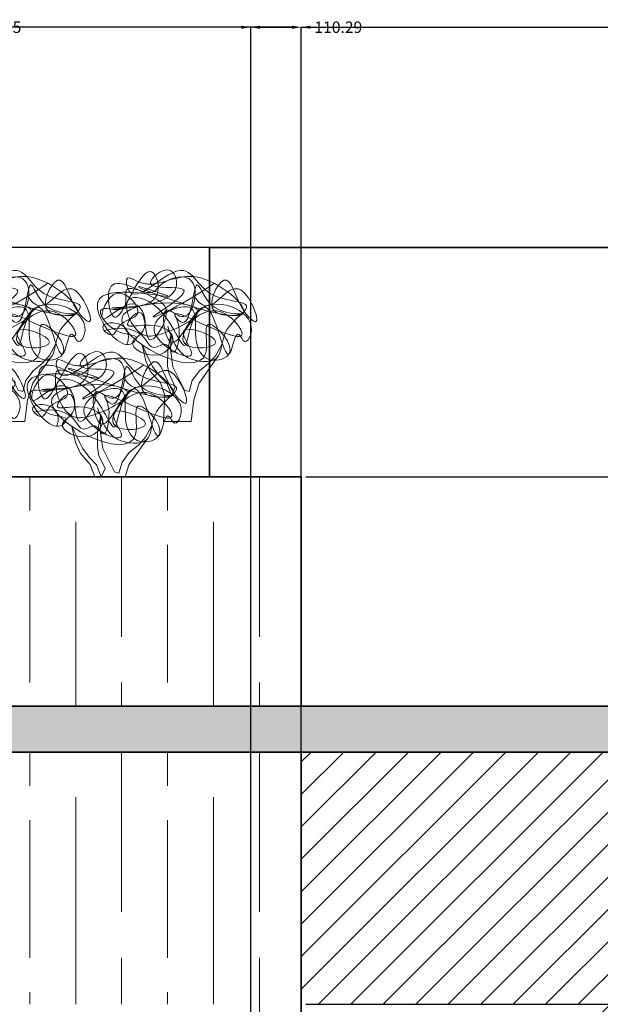
# Model space of a CAD drawing. Units: millimetres. Extents: x -692 to 9639, y -141 to 10345.
# Tile 17 of 19: x 4578 to 5843, y 8199 to 10345. Entities that reach past the tile are written whole.
import ezdxf

# ---------------------------------------------------------------- set-up
doc = ezdxf.new("R2010")
doc.units = ezdxf.units.MM
doc.header["$MEASUREMENT"] = 0
for name, color, linetype, lineweight in [('A-ANNO-DIMS', 2, 'Continuous', 18), ('A-ELEV', 7, 'Continuous', 35), ('A-ELEV-PATT', 8, 'Continuous', 13), ('L-PLNT', 3, 'Continuous', 18)]:
    doc.layers.add(name, color=color, linetype=linetype, lineweight=lineweight)
doc.styles.get("Standard").update_dxf_attribs({"font": 'arial.ttf'})
doc.dimstyles.get("Standard").update_dxf_attribs({"dimtxt": 25, "dimasz": 20, "dimexe": 0.18, "dimexo": 10, "dimgap": 10, "dimtad": 0, "dimtih": 1, "dimtoh": 1, "dimdec": 0, "dimzin": 0, "dimdsep": 46, "dimtxsty": 'Standard', "dimcen": 10, "dimadec": 0, "dimazin": 0, "dimtfac": 1, "dimtdec": 0, "dimtofl": 0, "dimtmove": 0, "dimatfit": 3, "dimfxl": 1, "dimtolj": 1, "dimtzin": 0, "dimarcsym": 0})

# ---------------------------------------------------------------- blocks, each defined once
blk = doc.blocks.new('SHRUB-A')
for p, q in [((56.2, 156.7), (63.1, 192.4)), ((63.1, 192.4), (61.6, 157.6)), ((4.3, 148.6), (0, 167.6)), ((0, 167.6), (10, 146.8)), ((55.6, 120.9), (56.2, 156.7)), ((61.6, 157.6), (67.3, 119.6)), ((160.6, 144.2), (174.3, 169.5)), ((7.9, 132.5), (4.3, 148.6)), ((17.8, 109.9), (7.9, 132.5)), ((10, 146.8), (18, 130.3)), ((18, 130.3), (22.9, 120.3)), ((162.4, 138.4), (124.4, 83.7)), ((145.1, 126.5), (160.6, 144.2)), ((40.2, 84.8), (17.8, 109.9)), ((22.9, 120.3), (37.4, 100.1)), ((59.1, 104.1), (55.6, 120.9)), ((67.3, 119.6), (83.9, 86)), ((109.4, 89.7), (124.8, 110.5)), ((124.8, 110.5), (145.1, 126.5)), ((37.4, 100.1), (54, 83.6)), ((72.4, 75.8), (59.1, 104.1)), ((83.9, 86), (92.7, 68.2)), ((102.6, 65.4), (109.4, 89.7)), ((49.7, 57.7), (40.2, 84.8)), ((54, 83.6), (64.1, 57.4)), ((64.1, 57.4), (72.4, 75.8)), ((92.7, 68.2), (102.6, 65.4)), ((124.4, 83.7), (113, 47.4)), ((47, 0.4), (49.7, 57.7)), ((113, 47.4), (106.7, 0)), ((106.7, 0), (47, 0.4))]:
    blk.add_line(p, q)
blk = doc.blocks.new('SHRUB-B')
for p, q in [((56.2, 99.2), (63.1, 135)), ((63.1, 135), (61.6, 100.2)), ((4.3, 91.2), (0, 110.2)), ((0, 110.2), (10, 89.4)), ((160.6, 86.8), (174.3, 112.1)), ((7.9, 75.1), (4.3, 91.2)), ((10, 89.4), (18, 72.9)), ((55.6, 63.5), (56.2, 99.2)), ((61.6, 100.2), (67.3, 62.2)), ((145.1, 69.1), (160.6, 86.8)), ((17.8, 52.5), (7.9, 75.1)), ((18, 72.9), (22.9, 62.9)), ((124.8, 53.1), (145.1, 69.1)), ((40.2, 27.4), (17.8, 52.5)), ((22.9, 62.9), (37.4, 42.7)), ((59.1, 46.7), (55.6, 63.5)), ((72.4, 18.4), (59.1, 46.7)), ((67.3, 62.2), (83.9, 28.6)), ((109.4, 32.3), (124.8, 53.1)), ((37.4, 42.7), (54, 26.2)), ((49.7, 0.3), (40.2, 27.4)), ((54, 26.2), (64.1, 0)), ((83.9, 28.6), (92.7, 10.8)), ((102.6, 8), (109.4, 32.3)), ((64.1, 0), (72.4, 18.4)), ((92.7, 10.8), (102.6, 8))]:
    blk.add_line(p, q)
blk = doc.blocks.new('*D7')
at = {"layer": 'A-ANNO-DIMS', "color": 0, "lineweight": -2, "transparency": 16777216}
for p, q in [((8481.5, 9848.8), (-649.1, 9848.8)), ((-648.9, 9828.8), (-648.9, 5124.9)), ((-648.9, 375.6), (-648.9, 5079.4)), ((2463.7, 355.6), (-649.1, 355.6))]:
    blk.add_line(p, q, dxfattribs=at)
at = {"layer": 'A-ANNO-DIMS', "color": 0, "lineweight": -3, "transparency": 16777216}
for points in [[(-652.2, 9828.8), (-645.6, 9828.8), (-648.9, 9848.8)], [(-652.2, 375.6), (-645.6, 375.6), (-648.9, 355.6)]]:
    blk.add_solid(points, dxfattribs=at)
at = {"layer": 'Defpoints', "color": 0, "lineweight": -3, "transparency": 16777216}
for p in [(-648.9, 9848.8), (8491.5, 9848.8), (2473.7, 355.6)]:
    blk.add_point(p, dxfattribs=at)
at = {"layer": 'A-ANNO-DIMS', "color": 0, "transparency": 16777216, "insert": (-648.9, 5102.2), "char_height": 25, "attachment_point": 5}
blk.add_mtext('\\A1;9493', dxfattribs=at)
blk = doc.blocks.new('*D11')
at = {"layer": 'A-ANNO-DIMS', "color": 0, "lineweight": -2, "transparency": 16777216}
for p, q in [((9553.7, 9348.8), (9553.7, 9368.8)), ((9553.7, 9368.8), (9573.7, 9368.8)), ((5201.5, 9348.8), (9553.9, 9348.8)), ((9553.7, 9268.8), (9553.7, 9328.8)), ((8251.5, 9248.8), (9553.9, 9248.8))]:
    blk.add_line(p, q, dxfattribs=at)
at = {"layer": 'A-ANNO-DIMS', "color": 0, "lineweight": -3, "transparency": 16777216}
for points in [[(9550.4, 9328.8), (9557.1, 9328.8), (9553.7, 9348.8)], [(9550.4, 9268.8), (9557.1, 9268.8), (9553.7, 9248.8)]]:
    blk.add_solid(points, dxfattribs=at)
at = {"layer": 'Defpoints', "color": 0, "lineweight": -3, "transparency": 16777216}
for p in [(5191.5, 9348.8), (9553.7, 9348.8), (8241.5, 9248.8)]:
    blk.add_point(p, dxfattribs=at)
at = {"layer": 'A-ANNO-DIMS', "color": 0, "transparency": 16777216, "insert": (9610.1, 9368.8), "char_height": 25, "attachment_point": 5}
blk.add_mtext('\\A1;100', dxfattribs=at)
blk = doc.blocks.new('*D12')
at = {"layer": 'A-ANNO-DIMS', "color": 0, "lineweight": -2, "transparency": 16777216}
for p, q in [((8251.5, 9598.8), (9553.9, 9598.8)), ((9553.7, 9578.8), (9553.7, 9496.5)), ((9553.7, 9368.8), (9553.7, 9451)), ((5201.5, 9348.8), (9553.9, 9348.8))]:
    blk.add_line(p, q, dxfattribs=at)
at = {"layer": 'A-ANNO-DIMS', "color": 0, "lineweight": -3, "transparency": 16777216}
for points in [[(9550.4, 9578.8), (9557.1, 9578.8), (9553.7, 9598.8)], [(9550.4, 9368.8), (9557.1, 9368.8), (9553.7, 9348.8)]]:
    blk.add_solid(points, dxfattribs=at)
at = {"layer": 'Defpoints', "color": 0, "lineweight": -3, "transparency": 16777216}
for p in [(8241.5, 9598.8), (9553.7, 9598.8), (5191.5, 9348.8)]:
    blk.add_point(p, dxfattribs=at)
at = {"layer": 'A-ANNO-DIMS', "color": 0, "transparency": 16777216, "insert": (9553.7, 9473.8), "char_height": 25, "attachment_point": 5}
blk.add_mtext('\\A1;250', dxfattribs=at)
blk = doc.blocks.new('*D14')
at = {"layer": 'A-ANNO-DIMS', "color": 0, "lineweight": -2, "transparency": 16777216}
for p, q in [((3191.5, 9358.8), (3191.5, 10329)), ((3211.5, 10328.8), (4144, 10328.8)), ((5171.5, 10328.8), (4239, 10328.8)), ((5191.5, 9358.8), (5191.5, 10329))]:
    blk.add_line(p, q, dxfattribs=at)
at = {"layer": 'A-ANNO-DIMS', "color": 0, "lineweight": -3, "transparency": 16777216}
for points in [[(3211.5, 10332.1), (3211.5, 10325.4), (3191.5, 10328.8)], [(5171.5, 10332.1), (5171.5, 10325.4), (5191.5, 10328.8)]]:
    blk.add_solid(points, dxfattribs=at)
at = {"layer": 'Defpoints', "color": 0, "lineweight": -3, "transparency": 16777216}
for p in [(5191.5, 10328.8), (3191.5, 9348.8), (5191.5, 9348.8)]:
    blk.add_point(p, dxfattribs=at)
at = {"layer": 'A-ANNO-DIMS', "color": 0, "transparency": 16777216, "insert": (4191.5, 10328.8), "char_height": 25, "attachment_point": 5}
blk.add_mtext('\\A1;2000', dxfattribs=at)
blk = doc.blocks.new('*D15')
at = {"layer": 'A-ANNO-DIMS', "color": 0, "lineweight": -2, "transparency": 16777216}
for p, q in [((5191.5, 9358.8), (5191.5, 10329)), ((5211.5, 10328.8), (5920.4, 10328.8)), ((6721.5, 10328.8), (6012.7, 10328.8)), ((6741.5, 9258.8), (6741.5, 10329))]:
    blk.add_line(p, q, dxfattribs=at)
at = {"layer": 'A-ANNO-DIMS', "color": 0, "lineweight": -3, "transparency": 16777216}
for points in [[(5211.5, 10332.1), (5211.5, 10325.4), (5191.5, 10328.8)], [(6721.5, 10332.1), (6721.5, 10325.4), (6741.5, 10328.8)]]:
    blk.add_solid(points, dxfattribs=at)
at = {"layer": 'Defpoints', "color": 0, "lineweight": -3, "transparency": 16777216}
for p in [(6741.5, 10328.8), (5191.5, 9348.8), (6741.5, 9248.8)]:
    blk.add_point(p, dxfattribs=at)
at = {"layer": 'A-ANNO-DIMS', "color": 0, "transparency": 16777216, "insert": (5966.5, 10328.8), "char_height": 25, "attachment_point": 5}
blk.add_mtext('\\A1;1550', dxfattribs=at)
blk = doc.blocks.new('*D54')
at = {"layer": 'A-ANNO-DIMS', "color": 0, "lineweight": -2, "transparency": 16777216}
for p, q in [((4006.3, 6433.8), (4006.3, 10329)), ((4026.3, 10328.8), (4497.5, 10328.8)), ((5061.3, 10328.8), (4590, 10328.8)), ((5081.3, 6433.8), (5081.3, 10329))]:
    blk.add_line(p, q, dxfattribs=at)
at = {"layer": 'A-ANNO-DIMS', "color": 0, "lineweight": -3, "transparency": 16777216}
for points in [[(4026.3, 10332.1), (4026.3, 10325.4), (4006.3, 10328.8)], [(5061.3, 10332.1), (5061.3, 10325.4), (5081.3, 10328.8)]]:
    blk.add_solid(points, dxfattribs=at)
at = {"layer": 'Defpoints', "color": 0, "lineweight": -3, "transparency": 16777216}
for p in [(5081.3, 10328.8), (4006.3, 6423.8), (5081.3, 6423.8)]:
    blk.add_point(p, dxfattribs=at)
at = {"layer": 'A-ANNO-DIMS', "color": 0, "transparency": 16777216, "insert": (4543.8, 10328.8), "char_height": 25, "attachment_point": 5}
blk.add_mtext('\\A1;1075', dxfattribs=at)
blk = doc.blocks.new('*D55')
at = {"layer": 'A-ANNO-DIMS', "color": 0, "lineweight": -2, "transparency": 16777216}
for p, q in [((5081.3, 6433.8), (5081.3, 10329)), ((5101.3, 10328.8), (5171.5, 10328.8)), ((5191.5, 6358.8), (5191.5, 10329)), ((5191.5, 10328.8), (5211.5, 10328.8))]:
    blk.add_line(p, q, dxfattribs=at)
at = {"layer": 'A-ANNO-DIMS', "color": 0, "lineweight": -3, "transparency": 16777216}
for points in [[(5101.3, 10332.1), (5101.3, 10325.4), (5081.3, 10328.8)], [(5171.5, 10332.1), (5171.5, 10325.4), (5191.5, 10328.8)]]:
    blk.add_solid(points, dxfattribs=at)
at = {"layer": 'Defpoints', "color": 0, "lineweight": -3, "transparency": 16777216}
for p in [(5191.5, 10328.8), (5081.3, 6423.8), (5191.5, 6348.8)]:
    blk.add_point(p, dxfattribs=at)
at = {"layer": 'A-ANNO-DIMS', "color": 0, "transparency": 16777216, "insert": (5272.3, 10328.8), "char_height": 25, "attachment_point": 5}
blk.add_mtext('\\A1;110.29', dxfattribs=at)
blk = doc.blocks.new('*D56')
at = {"layer": 'A-ANNO-DIMS', "color": 0, "lineweight": -2, "transparency": 16777216}
for p, q in [((5191.5, 6358.8), (5191.5, 10329)), ((5211.5, 10328.8), (5981.1, 10328.8)), ((6871.7, 10328.8), (6102.2, 10328.8)), ((6891.7, 6708.8), (6891.7, 10329))]:
    blk.add_line(p, q, dxfattribs=at)
at = {"layer": 'A-ANNO-DIMS', "color": 0, "lineweight": -3, "transparency": 16777216}
for points in [[(5211.5, 10332.1), (5211.5, 10325.4), (5191.5, 10328.8)], [(6871.7, 10332.1), (6871.7, 10325.4), (6891.7, 10328.8)]]:
    blk.add_solid(points, dxfattribs=at)
at = {"layer": 'Defpoints', "color": 0, "lineweight": -3, "transparency": 16777216}
for p in [(6891.7, 10328.8), (6891.7, 6698.8), (5191.5, 6348.8)]:
    blk.add_point(p, dxfattribs=at)
at = {"layer": 'A-ANNO-DIMS', "color": 0, "transparency": 16777216, "insert": (6041.6, 10328.8), "char_height": 25, "attachment_point": 5}
blk.add_mtext('\\A1;1700.2', dxfattribs=at)
blk = doc.blocks.new('*D77')
at = {"layer": 'A-ANNO-DIMS', "color": 0, "lineweight": -2, "transparency": 16777216}
for p, q in [((5201.5, 8198.8), (9553.9, 8198.8)), ((9553.7, 8178.8), (9553.7, 7771.8)), ((9553.7, 7319.3), (9553.7, 7726.3)), ((5201.5, 7299.3), (9553.9, 7299.3))]:
    blk.add_line(p, q, dxfattribs=at)
at = {"layer": 'A-ANNO-DIMS', "color": 0, "lineweight": -3, "transparency": 16777216}
for points in [[(9550.4, 8178.8), (9557.1, 8178.8), (9553.7, 8198.8)], [(9550.4, 7319.3), (9557.1, 7319.3), (9553.7, 7299.3)]]:
    blk.add_solid(points, dxfattribs=at)
at = {"layer": 'Defpoints', "color": 0, "lineweight": -3, "transparency": 16777216}
for p in [(5191.5, 8198.8), (9553.7, 8198.8), (5191.5, 7299.3)]:
    blk.add_point(p, dxfattribs=at)
at = {"layer": 'A-ANNO-DIMS', "color": 0, "transparency": 16777216, "insert": (9553.7, 7749), "char_height": 25, "attachment_point": 5}
blk.add_mtext('\\A1;899.5', dxfattribs=at)
blk = doc.blocks.new('*D78')
at = {"layer": 'A-ANNO-DIMS', "color": 0, "lineweight": -2, "transparency": 16777216}
for p, q in [((8401.5, 8748.8), (9553.9, 8748.8)), ((9553.7, 8728.8), (9553.7, 8496.5)), ((9553.7, 8218.8), (9553.7, 8451)), ((5201.5, 8198.8), (9553.9, 8198.8))]:
    blk.add_line(p, q, dxfattribs=at)
at = {"layer": 'A-ANNO-DIMS', "color": 0, "lineweight": -3, "transparency": 16777216}
for points in [[(9550.4, 8728.8), (9557.1, 8728.8), (9553.7, 8748.8)], [(9550.4, 8218.8), (9557.1, 8218.8), (9553.7, 8198.8)]]:
    blk.add_solid(points, dxfattribs=at)
at = {"layer": 'Defpoints', "color": 0, "lineweight": -3, "transparency": 16777216}
for p in [(8391.5, 8748.8), (9553.7, 8748.8), (5191.5, 8198.8)]:
    blk.add_point(p, dxfattribs=at)
at = {"layer": 'A-ANNO-DIMS', "color": 0, "transparency": 16777216, "insert": (9553.7, 8473.8), "char_height": 25, "attachment_point": 5}
blk.add_mtext('\\A1;550', dxfattribs=at)

msp = doc.modelspace()

# ---------------------------------------------------------------- hatches: boundary and pattern name
at = {"layer": 'A-ELEV-PATT'}
h = msp.add_hatch(dxfattribs=at)
h.set_pattern_fill('GOST_WOOD', color=256, scale=50)
h.set_pattern_definition([(90, (0, 0), (300, -2e-14), [500, -100]), (90, (100, -100), (300, -2e-14), [300, -75, 150, -75]), (90, (200, -250), (300, -2e-14), [500, -100])])
edge = h.paths.add_edge_path()
edge.add_line((5191.547, 8748.772), (3791.547, 8748.772))
edge.add_line((3791.547, 8748.772), (3791.547, 8848.772))
edge.add_line((3791.547, 8848.772), (5191.547, 8848.772))
edge.add_line((5191.547, 8848.772), (5191.547, 9348.772))
edge.add_line((5191.547, 9348.772), (4755.992, 9348.772))
edge.add_line((4755.992, 9348.772), (4755.854, 9348.465))
edge.add_line((4755.854, 9348.465), (4755.734, 9348.772))
edge.add_line((4755.734, 9348.772), (4053.129, 9348.772))
edge.add_line((4053.129, 9348.772), (4052.99, 9348.465))
edge.add_line((4052.99, 9348.465), (4052.871, 9348.772))
edge.add_line((4052.871, 9348.772), (3701.731, 9348.772))
edge.add_line((3701.731, 9348.772), (3701.593, 9348.465))
edge.add_line((3701.593, 9348.465), (3701.474, 9348.772))
edge.add_line((3701.474, 9348.772), (3368.199, 9348.772))
edge.add_line((3368.199, 9348.772), (3368.061, 9348.465))
edge.add_line((3368.061, 9348.465), (3367.942, 9348.772))
edge.add_line((3367.942, 9348.772), (3191.547, 9348.772))
edge.add_line((3191.547, 9348.772), (3191.547, 3210.058))
edge.add_spline(control_points=[(3191.547, 3210.058), (3198.467, 3207.5), (3283.859, 3166.656), (3324.053, 2995.08), (3234.02, 2920.058), (3220.783, 2911.684)], knot_values=[13649.89756952, 13649.89756952, 13649.89756952, 13649.89756952, 13672.14990348, 13935.42377748, 13974.4426778, 13974.4426778, 13974.4426778, 13974.4426778], degree=3, periodic=0)
edge.add_spline(control_points=[(3220.783, 2911.684), (3225.148, 2890.107), (3226.864, 2868.931), (3226.144, 2848.27)], knot_values=[8828.69997321, 8828.69997321, 8828.69997321, 8828.69997321, 8890.6429847, 8890.6429847, 8890.6429847, 8890.6429847], degree=3, periodic=0)
edge.add_line((3226.144, 2848.27), (5191.547, 2848.27))
edge.add_line((5191.547, 2848.27), (5191.547, 3048.27))
edge.add_line((5191.547, 3048.27), (5041.547, 3048.27))
edge.add_line((5041.547, 3048.27), (5041.547, 3148.27))
edge.add_line((5041.547, 3148.27), (5091.547, 3148.27))
edge.add_line((5091.547, 3148.27), (5091.547, 3598.27))
edge.add_line((5091.547, 3598.27), (5191.547, 3598.27))
edge.add_line((5191.547, 3598.27), (5191.547, 4848.772))
edge.add_line((5191.547, 4848.772), (3791.547, 4848.772))
edge.add_line((3791.547, 4848.772), (3791.547, 6848.772))
edge.add_line((3791.547, 6848.772), (5091.547, 6848.772))
edge.add_line((5091.547, 6848.772), (5091.547, 7298.772))
edge.add_line((5091.547, 7298.772), (5191.547, 7298.772))
edge.add_line((5191.547, 7298.772), (5191.547, 8748.772))
h.paths.add_polyline_path([(5016.547, 8198.772), (5016.547, 7123.772), (3941.547, 7123.772), (3941.547, 8198.772)], flags=16)
h.paths.add_polyline_path([(4941.547, 8123.772), (4941.547, 7198.772), (4016.547, 7198.772), (4016.547, 8123.772)], flags=0)
h.paths.add_polyline_path([(4616.547, 8073.772), (4616.547, 7248.772), (4341.547, 7248.772), (4341.547, 8073.772)], flags=0)
h.paths.add_polyline_path([(4641.547, 8073.772), (4891.547, 8073.772), (4891.547, 7248.772), (4641.547, 7248.772)], flags=0)
h.paths.add_polyline_path([(4666.547, 8048.772), (4866.547, 8048.772), (4866.547, 7273.772), (4666.547, 7273.772)], flags=0)
h.paths.add_polyline_path([(4316.547, 8073.772), (4316.547, 7248.772), (4066.547, 7248.772), (4066.547, 8073.772)], flags=0)
h.paths.add_polyline_path([(4291.547, 8048.772), (4291.547, 7273.772), (4091.547, 7273.772), (4091.547, 8048.772)], flags=0)
h.paths.add_polyline_path([(5016.547, 4497.772), (5016.547, 3422.772), (3941.547, 3422.772), (3941.547, 4497.772)], flags=16)
h.paths.add_polyline_path([(4941.547, 4422.772), (4941.547, 3497.772), (4016.547, 3497.772), (4016.547, 4422.772)], flags=0)
h.paths.add_polyline_path([(4616.547, 4372.772), (4616.547, 3547.772), (4341.547, 3547.772), (4341.547, 4372.772)], flags=0)
h.paths.add_polyline_path([(4641.547, 4372.772), (4891.547, 4372.772), (4891.547, 3547.772), (4641.547, 3547.772)], flags=0)
h.paths.add_polyline_path([(4316.547, 4372.772), (4316.547, 3547.772), (4066.547, 3547.772), (4066.547, 4372.772)], flags=0)
h.paths.add_polyline_path([(4666.547, 4347.772), (4866.547, 4347.772), (4866.547, 3572.772), (4666.547, 3572.772)], flags=0)
h.paths.add_polyline_path([(4291.547, 4347.772), (4291.547, 3572.772), (4091.547, 3572.772), (4091.547, 4347.772)], flags=0)
h = msp.add_hatch(dxfattribs=at)
h.set_pattern_fill('CROSS', color=256, scale=150)
h.paths.add_polyline_path([(8491.547, 8848.772), (3791.547, 8848.772), (3791.547, 8748.772), (8391.547, 8748.772), (8391.547, 6848.772), (8491.547, 6848.772)])
h = msp.add_hatch(dxfattribs=at)
h.set_pattern_fill('ANSI31', color=256, scale=400)
h.paths.add_polyline_path([(6891.746, 6698.772), (5191.547, 6698.772), (5191.547, 6348.772), (5841.547, 6348.772), (5841.547, 5448.772), (6041.547, 5448.772), (6041.547, 6348.772), (6691.547, 6348.772), (6691.547, 5448.772), (6891.746, 5448.772)])
h.paths.add_polyline_path([(5191.547, 6698.772), (3941.547, 6698.772), (3941.547, 5448.772), (4006.259, 5448.772), (4006.259, 6423.772), (5081.259, 6423.772), (5081.259, 5448.772), (5191.547, 5448.772), (5191.547, 6348.772)])
h.paths.add_polyline_path([(6891.746, 4848.772), (5191.547, 4848.772), (5191.547, 4497.772), (5841.746, 4497.772), (5841.746, 3598.27), (6041.746, 3598.27), (6041.746, 4497.772), (6691.746, 4497.772), (6691.746, 3598.27), (6891.746, 3598.27)])
h.paths.add_polyline_path([(6891.746, 8748.772), (5191.547, 8748.772), (5191.547, 8198.772), (5841.547, 8198.772), (5841.547, 7298.772), (6041.547, 7298.772), (6041.547, 8198.772), (6691.547, 8198.772), (6691.547, 7298.772), (6891.746, 7298.772)])

# ---------------------------------------------------------------- linework, layer by layer
at = {"layer": 'A-ELEV'}
for p, q in [((8491.547, 9848.772), (4991.547, 9848.772)), ((4991.547, 9848.772), (4991.547, 9348.772)), ((3191.547, 9348.772), (5191.547, 9348.772)), ((5191.547, 9348.772), (5191.547, 8848.772)), ((3791.547, 8848.772), (8491.547, 8848.772)), ((3791.547, 8748.772), (8391.547, 8748.772)), ((5191.547, 7298.772), (5191.547, 8748.772))]:
    msp.add_line(p, q, dxfattribs=at)
at = {"layer": 'L-PLNT'}
for p, q in [((4854.157, 9429.44), (4816.092, 9374.709)), ((4816.092, 9374.709), (4808.516, 9350.541))]:
    msp.add_line(p, q, dxfattribs=at)
for points, knots in [([(4595.897, 9742.239), (4602.402, 9730.903), (4635.638, 9700.951), (4692.068, 9812.559), (4751.248, 9660.867), (4686.612, 9722.363), (4670.887, 9821.568), (4603.928, 9687.955), (4741.394, 9708.276), (4624.549, 9697.909), (4595.213, 9822.951), (4589.611, 9656.273), (4537.109, 9718.176), (4630.79, 9672.588), (4727.856, 9634.5), (4658.695, 9723.816), (4592.541, 9704.087), (4550.33, 9620.458), (4701.218, 9634.855), (4535.609, 9696.668), (4631.983, 9576.858), (4438.141, 9670.533), (4612.837, 9749.582), (4590.628, 9651.408), (4619.366, 9592.145), (4705.618, 9617.027), (4603.784, 9721.539), (4658.99, 9522.359), (4273.396, 9733.486), (4688.49, 9736.751), (4538.507, 9659.817), (4467.655, 9649.423), (4424.843, 9757.262), (4539.624, 9723.536), (4581.712, 9579.097), (4586.697, 9768.661), (4748.391, 9702.629), (4705.664, 9633.263), (4687.627, 9680.84), (4666.832, 9544.945), (4630.078, 9826.86), (4542.947, 9563.572), (4517.945, 9739.876), (4587.714, 9668.929), (4619.381, 9809.339), (4528.84, 9778.979), (4499.715, 9737.949), (4432.772, 9784.348), (4458.963, 9697.774), (4366.521, 9733.91), (4416.338, 9654.8), (4477.857, 9658.957), (4447.691, 9620.328), (4392.387, 9675.174), (4368.105, 9782.065), (4612.479, 9719.852), (4364.188, 9801.027), (4824.937, 9622.054), (4599.272, 9821.297), (4519.429, 9760.575), (4473.126, 9773.261), (4445.042, 9789.116), (4457.404, 9699.252), (4558.733, 9839.527), (4610.872, 9759.776), (4649.687, 9734.293), (4741.363, 9726.404), (4648.346, 9674.075), (4662.506, 9593.308), (4562.689, 9601.408), (4547.062, 9650.09), (4538.319, 9677.329)], [2413.81083439, 2413.81083439, 2413.81083439, 2413.81083439, 2446.13175162, 2525.76080664, 2606.35842411, 2641.00152553, 2720.74212251, 2790.99014926, 2851.81652626, 2913.32865241, 2976.26621652, 3063.90114016, 3082.75198237, 3142.42040078, 3234.21047015, 3290.89514405, 3366.44484787, 3415.98940505, 3483.69911772, 3557.93307926, 3609.73318023, 3705.73947781, 3799.4035149, 3865.9559372, 3923.0506034, 3967.47996902, 4044.49288828, 4106.44083814, 4304.51898163, 4470.20683119, 4567.66187689, 4605.3795614, 4686.71522755, 4750.59418277, 4853.67923318, 4940.38216709, 5061.92671957, 5081.75583403, 5102.38342504, 5145.20608443, 5257.20859169, 5364.77120979, 5434.601162, 5468.93345211, 5548.91442162, 5624.29444335, 5636.24531967, 5696.20028889, 5735.53268567, 5783.76480276, 5846.42206129, 5886.03768999, 5892.5373904, 5975.51315878, 6025.10951571, 6171.93373357, 6229.50952465, 6457.88730992, 6585.61219414, 6694.59236697, 6720.94216912, 6740.48817363, 6762.80712224, 6890.45590486, 6938.76737224, 6996.52597549, 7050.2147859, 7119.04318667, 7183.57042671, 7247.02609863, 7327.63038966, 7327.63038966, 7327.63038966, 7327.63038966]), ([(4449.206, 9637.137), (4455.269, 9651.341), (4451.774, 9689.445), (4377.203, 9684.583), (4420.651, 9647.305), (4431.332, 9691.38), (4500.393, 9694.456), (4420.441, 9786.768), (4371.946, 9649.897), (4470.421, 9765.156), (4502.196, 9667.558), (4438.143, 9636.75), (4520.946, 9595.485), (4568.292, 9663.04), (4503.846, 9686.864), (4433.305, 9669.411), (4494.809, 9738.522), (4481.865, 9597.689), (4556.176, 9714.368), (4490.412, 9747.322), (4394.637, 9801.44), (4418.802, 9656.882), (4458.375, 9753.527), (4505.512, 9818.105), (4539.103, 9708.231), (4310.355, 9723.215), (4584.503, 9710.208), (4544.502, 9819.441), (4461.103, 9748.74), (4636.137, 9777.439), (4424.613, 9652.419), (4588.866, 9733.103), (4638.998, 9770.678)], [369.05069933, 369.05069933, 369.05069933, 369.05069933, 408.0755152, 451.81999766, 477.70991819, 501.76804774, 551.72688153, 614.71506468, 677.59190345, 752.65992621, 814.92518896, 848.06947292, 911.78367098, 957.89252981, 1028.01014559, 1063.15062915, 1099.93333455, 1162.00574744, 1235.23981988, 1278.45742209, 1371.86548038, 1434.47491944, 1513.90135623, 1562.79289697, 1613.81915843, 1716.27616866, 1864.9556669, 1902.31221643, 1951.61463942, 2025.20033993, 2111.30740148, 2244.75178922, 2244.75178922, 2244.75178922, 2244.75178922]), ([(4958.34, 9742.239), (4964.846, 9730.903), (4998.082, 9700.951), (5054.512, 9812.559), (5113.692, 9660.867), (5049.056, 9722.363), (5033.33, 9821.568), (4966.371, 9687.955), (5103.837, 9708.276), (4986.993, 9697.909), (4957.657, 9822.951), (4952.055, 9656.273), (4899.553, 9718.176), (4993.234, 9672.588), (5090.299, 9634.5), (5021.138, 9723.816), (4954.985, 9704.087), (4912.774, 9620.458), (5063.661, 9634.855), (4898.053, 9696.668), (4994.427, 9576.858), (4800.585, 9670.533), (4975.281, 9749.582), (4953.072, 9651.408), (4981.81, 9592.145), (5068.062, 9617.027), (4966.228, 9721.539), (5021.434, 9522.359), (4635.84, 9733.486), (5050.934, 9736.751), (4900.951, 9659.817), (4830.099, 9649.423), (4787.287, 9757.262), (4902.068, 9723.536), (4944.155, 9579.097), (4949.141, 9768.661), (5110.834, 9702.629), (5068.107, 9633.263), (5050.07, 9680.84), (5029.275, 9544.945), (4992.522, 9826.86), (4905.39, 9563.572), (4880.389, 9739.876), (4950.157, 9668.929), (4981.824, 9809.339), (4891.284, 9778.979), (4862.158, 9737.949), (4795.216, 9784.348), (4821.407, 9697.774), (4728.965, 9733.91), (4778.781, 9654.8), (4840.301, 9658.957), (4810.134, 9620.328), (4754.83, 9675.174), (4730.549, 9782.065), (4974.923, 9719.852), (4726.631, 9801.027), (5187.381, 9622.054), (4961.716, 9821.297), (4881.872, 9760.575), (4835.57, 9773.261), (4807.486, 9789.116), (4819.848, 9699.252), (4921.176, 9839.527), (4973.316, 9759.776), (5012.13, 9734.293), (5103.806, 9726.404), (5010.789, 9674.075), (5024.95, 9593.308), (4925.132, 9601.408), (4909.506, 9650.09), (4900.762, 9677.329)], [2413.81083439, 2413.81083439, 2413.81083439, 2413.81083439, 2446.13175162, 2525.76080664, 2606.35842411, 2641.00152553, 2720.74212251, 2790.99014926, 2851.81652626, 2913.32865241, 2976.26621652, 3063.90114016, 3082.75198237, 3142.42040078, 3234.21047015, 3290.89514405, 3366.44484787, 3415.98940505, 3483.69911772, 3557.93307926, 3609.73318023, 3705.73947781, 3799.4035149, 3865.9559372, 3923.0506034, 3967.47996902, 4044.49288828, 4106.44083814, 4304.51898163, 4470.20683119, 4567.66187689, 4605.3795614, 4686.71522755, 4750.59418277, 4853.67923318, 4940.38216709, 5061.92671957, 5081.75583403, 5102.38342504, 5145.20608443, 5257.20859169, 5364.77120979, 5434.601162, 5468.93345211, 5548.91442162, 5624.29444335, 5636.24531967, 5696.20028889, 5735.53268567, 5783.76480276, 5846.42206129, 5886.03768999, 5892.5373904, 5975.51315878, 6025.10951571, 6171.93373357, 6229.50952465, 6457.88730992, 6585.61219414, 6694.59236697, 6720.94216912, 6740.48817363, 6762.80712224, 6890.45590486, 6938.76737224, 6996.52597549, 7050.2147859, 7119.04318667, 7183.57042671, 7247.02609863, 7327.63038966, 7327.63038966, 7327.63038966, 7327.63038966]), ([(4811.649, 9637.137), (4817.712, 9651.341), (4814.218, 9689.445), (4739.647, 9684.583), (4783.094, 9647.305), (4793.776, 9691.38), (4862.837, 9694.456), (4782.885, 9786.768), (4734.39, 9649.897), (4832.865, 9765.156), (4864.64, 9667.558), (4800.587, 9636.75), (4883.39, 9595.485), (4930.736, 9663.04), (4866.29, 9686.864), (4795.748, 9669.411), (4857.253, 9738.522), (4844.308, 9597.689), (4918.62, 9714.368), (4852.856, 9747.322), (4757.08, 9801.44), (4781.245, 9656.882), (4820.819, 9753.527), (4867.955, 9818.105), (4901.546, 9708.231), (4672.798, 9723.215), (4946.947, 9710.208), (4906.945, 9819.441), (4823.546, 9748.74), (4998.581, 9777.439), (4787.057, 9652.419), (4951.31, 9733.103), (5001.441, 9770.678)], [369.05069933, 369.05069933, 369.05069933, 369.05069933, 408.0755152, 451.81999766, 477.70991819, 501.76804774, 551.72688153, 614.71506468, 677.59190345, 752.65992621, 814.92518896, 848.06947292, 911.78367098, 957.89252981, 1028.01014559, 1063.15062915, 1099.93333455, 1162.00574744, 1235.23981988, 1278.45742209, 1371.86548038, 1434.47491944, 1513.90135623, 1562.79289697, 1613.81915843, 1716.27616866, 1864.9556669, 1902.31221643, 1951.61463942, 2025.20033993, 2111.30740148, 2244.75178922, 2244.75178922, 2244.75178922, 2244.75178922]), ([(4916.37, 9700.071), (4919.86, 9693.404), (4931.357, 9671.444), (4918.286, 9597.516), (4897.105, 9646.949), (4864.295, 9618.501), (4846.708, 9674.749), (4788.955, 9675.405), (4762.243, 9667.541)], [0, 0, 0, 0, 24.87287104, 81.92705424, 103.09014331, 128.64171207, 165.87657864, 231.33124244, 231.33124244, 231.33124244, 231.33124244]), ([(4454.121, 9574.89), (4460.627, 9563.555), (4493.863, 9533.603), (4550.293, 9645.211), (4609.473, 9493.518), (4544.837, 9555.014), (4529.111, 9654.219), (4462.152, 9520.607), (4599.618, 9540.927), (4482.774, 9530.56), (4453.438, 9655.602), (4447.835, 9488.925), (4395.334, 9550.827), (4489.014, 9505.239), (4586.08, 9467.152), (4516.919, 9556.467), (4450.766, 9536.738), (4408.555, 9453.11), (4559.442, 9467.506), (4393.833, 9529.319), (4490.208, 9409.509), (4296.366, 9503.184), (4471.062, 9582.233), (4448.853, 9484.06), (4477.59, 9424.796), (4563.843, 9449.679), (4462.009, 9554.19), (4517.215, 9355.01), (4131.621, 9566.137), (4546.715, 9569.402), (4396.732, 9492.468), (4325.88, 9482.075), (4283.067, 9589.914), (4397.848, 9556.187), (4439.936, 9411.748), (4444.922, 9601.313), (4606.615, 9535.28), (4563.888, 9465.914), (4545.851, 9513.492), (4525.056, 9377.596), (4488.303, 9659.511), (4401.171, 9396.224), (4376.169, 9572.528), (4445.938, 9501.581), (4477.605, 9641.99), (4387.065, 9611.631), (4357.939, 9570.6), (4290.997, 9617), (4317.188, 9530.425), (4224.746, 9566.561), (4274.562, 9487.452), (4336.082, 9491.609), (4305.915, 9452.98), (4250.611, 9507.825), (4226.33, 9614.716), (4470.704, 9552.503), (4222.412, 9633.678), (4683.161, 9454.705), (4457.497, 9653.948), (4377.653, 9593.226), (4331.351, 9605.912), (4303.267, 9621.768), (4315.629, 9531.903), (4416.957, 9672.178), (4469.097, 9592.428), (4507.911, 9566.944), (4599.587, 9559.055), (4506.57, 9506.727), (4520.731, 9425.959), (4420.913, 9434.059), (4405.287, 9482.742), (4396.543, 9509.98)], [2413.81083439, 2413.81083439, 2413.81083439, 2413.81083439, 2446.13175162, 2525.76080664, 2606.35842411, 2641.00152553, 2720.74212251, 2790.99014926, 2851.81652626, 2913.32865241, 2976.26621652, 3063.90114016, 3082.75198237, 3142.42040078, 3234.21047015, 3290.89514405, 3366.44484787, 3415.98940505, 3483.69911772, 3557.93307926, 3609.73318023, 3705.73947781, 3799.4035149, 3865.9559372, 3923.0506034, 3967.47996902, 4044.49288828, 4106.44083814, 4304.51898163, 4470.20683119, 4567.66187689, 4605.3795614, 4686.71522755, 4750.59418277, 4853.67923318, 4940.38216709, 5061.92671957, 5081.75583403, 5102.38342504, 5145.20608443, 5257.20859169, 5364.77120979, 5434.601162, 5468.93345211, 5548.91442162, 5624.29444335, 5636.24531967, 5696.20028889, 5735.53268567, 5783.76480276, 5846.42206129, 5886.03768999, 5892.5373904, 5975.51315878, 6025.10951571, 6171.93373357, 6229.50952465, 6457.88730992, 6585.61219414, 6694.59236697, 6720.94216912, 6740.48817363, 6762.80712224, 6890.45590486, 6938.76737224, 6996.52597549, 7050.2147859, 7119.04318667, 7183.57042671, 7247.02609863, 7327.63038966, 7327.63038966, 7327.63038966, 7327.63038966]), ([(4805.38, 9564.196), (4811.886, 9552.861), (4845.122, 9522.909), (4901.551, 9634.516), (4960.732, 9482.824), (4896.096, 9544.32), (4880.37, 9643.525), (4813.411, 9509.913), (4950.877, 9530.233), (4834.032, 9519.866), (4804.697, 9644.908), (4799.094, 9478.231), (4746.592, 9540.133), (4840.273, 9494.545), (4937.339, 9456.457), (4868.178, 9545.773), (4802.025, 9526.044), (4759.813, 9442.416), (4910.701, 9456.812), (4745.092, 9518.625), (4841.466, 9398.815), (4647.624, 9492.49), (4822.321, 9571.539), (4800.112, 9473.365), (4828.849, 9414.102), (4915.102, 9438.984), (4813.268, 9543.496), (4868.473, 9344.316), (4482.88, 9555.443), (4897.973, 9558.708), (4747.99, 9481.774), (4677.139, 9471.381), (4634.326, 9579.22), (4749.107, 9545.493), (4791.195, 9401.054), (4796.181, 9590.618), (4957.874, 9524.586), (4915.147, 9455.22), (4897.11, 9502.798), (4876.315, 9366.902), (4839.561, 9648.817), (4752.43, 9385.529), (4727.428, 9561.834), (4797.197, 9490.886), (4828.864, 9631.296), (4738.324, 9600.937), (4709.198, 9559.906), (4642.256, 9606.306), (4668.446, 9519.731), (4576.005, 9555.867), (4625.821, 9476.758), (4687.341, 9480.914), (4657.174, 9442.286), (4601.87, 9497.131), (4577.588, 9604.022), (4821.963, 9541.809), (4573.671, 9622.984), (5034.42, 9444.011), (4808.756, 9643.254), (4728.912, 9582.532), (4682.609, 9595.218), (4654.525, 9611.073), (4666.887, 9521.209), (4768.216, 9661.484), (4820.356, 9581.734), (4859.17, 9556.25), (4950.846, 9548.361), (4857.829, 9496.032), (4871.99, 9415.265), (4772.172, 9423.365), (4756.546, 9472.047), (4747.802, 9499.286)], [2413.81083439, 2413.81083439, 2413.81083439, 2413.81083439, 2446.13175162, 2525.76080664, 2606.35842411, 2641.00152553, 2720.74212251, 2790.99014926, 2851.81652626, 2913.32865241, 2976.26621652, 3063.90114016, 3082.75198237, 3142.42040078, 3234.21047015, 3290.89514405, 3366.44484787, 3415.98940505, 3483.69911772, 3557.93307926, 3609.73318023, 3705.73947781, 3799.4035149, 3865.9559372, 3923.0506034, 3967.47996902, 4044.49288828, 4106.44083814, 4304.51898163, 4470.20683119, 4567.66187689, 4605.3795614, 4686.71522755, 4750.59418277, 4853.67923318, 4940.38216709, 5061.92671957, 5081.75583403, 5102.38342504, 5145.20608443, 5257.20859169, 5364.77120979, 5434.601162, 5468.93345211, 5548.91442162, 5624.29444335, 5636.24531967, 5696.20028889, 5735.53268567, 5783.76480276, 5846.42206129, 5886.03768999, 5892.5373904, 5975.51315878, 6025.10951571, 6171.93373357, 6229.50952465, 6457.88730992, 6585.61219414, 6694.59236697, 6720.94216912, 6740.48817363, 6762.80712224, 6890.45590486, 6938.76737224, 6996.52597549, 7050.2147859, 7119.04318667, 7183.57042671, 7247.02609863, 7327.63038966, 7327.63038966, 7327.63038966, 7327.63038966]), ([(4658.689, 9459.094), (4664.752, 9473.298), (4661.258, 9511.403), (4586.686, 9506.54), (4630.134, 9469.262), (4640.816, 9513.337), (4709.877, 9516.414), (4629.925, 9608.725), (4581.429, 9471.854), (4679.905, 9587.113), (4711.68, 9489.516), (4647.626, 9458.707), (4730.429, 9417.442), (4777.776, 9484.997), (4713.329, 9508.821), (4642.788, 9491.368), (4704.293, 9560.479), (4691.348, 9419.646), (4765.659, 9536.325), (4699.896, 9569.279), (4604.12, 9623.397), (4628.285, 9478.839), (4667.859, 9575.484), (4714.995, 9640.062), (4748.586, 9530.189), (4519.838, 9545.172), (4793.986, 9532.166), (4753.985, 9641.398), (4670.586, 9570.697), (4845.621, 9599.396), (4634.097, 9474.376), (4798.35, 9555.06), (4848.481, 9592.636)], [369.05069933, 369.05069933, 369.05069933, 369.05069933, 408.0755152, 451.81999766, 477.70991819, 501.76804774, 551.72688153, 614.71506468, 677.59190345, 752.65992621, 814.92518896, 848.06947292, 911.78367098, 957.89252981, 1028.01014559, 1063.15062915, 1099.93333455, 1162.00574744, 1235.23981988, 1278.45742209, 1371.86548038, 1434.47491944, 1513.90135623, 1562.79289697, 1613.81915843, 1716.27616866, 1864.9556669, 1902.31221643, 1951.61463942, 2025.20033993, 2111.30740148, 2244.75178922, 2244.75178922, 2244.75178922, 2244.75178922]), ([(4763.41, 9522.028), (4766.9, 9515.361), (4778.397, 9493.402), (4765.326, 9419.473), (4744.144, 9468.907), (4711.334, 9440.458), (4693.748, 9496.706), (4635.995, 9497.363), (4609.283, 9489.498)], [0, 0, 0, 0, 24.87287104, 81.92705424, 103.09014331, 128.64171207, 165.87657864, 231.33124244, 231.33124244, 231.33124244, 231.33124244])]:
    msp.add_open_spline(points, degree=3, knots=knots, dxfattribs=at)

# ---------------------------------------------------------------- block references
for name, p in [('SHRUB-A', (4482.228, 9469.1)), ('SHRUB-A', (4844.672, 9469.1)), ('SHRUB-B', (4691.712, 9348.465))]:
    msp.add_blockref(name, p, dxfattribs=at)

# ---------------------------------------------------------------- dimensions: what is measured, and where the dimension line sits
at = {"layer": 'A-ANNO-DIMS'}
for base, p1, p2, override, picture, middle in [((5191.547, 10328.772), (3191.547, 9348.772), (5191.547, 9348.772), {"dimdec": 0, "dimlfac": 1, "dimrnd": 0, "dimzin": 0, "dimdsep": 46, "dimlunit": 2}, '*D14', (4191.547, 10328.772)), ((5081.259, 10328.772), (4006.259, 6423.772), (5081.259, 6423.772), {"dimdec": 0, "dimlfac": 1, "dimrnd": 0, "dimzin": 0, "dimdsep": 46, "dimlunit": 2}, '*D54', (4543.759, 10328.772)), ((5191.547, 10328.772), (5081.259, 6423.772), (5191.547, 6348.772), {"dimdec": 2, "dimlfac": 1, "dimrnd": 0, "dimzin": 0, "dimdsep": 46, "dimlunit": 2}, '*D55', (5272.288, 10328.772)), ((6741.547, 10328.772), (5191.547, 9348.772), (6741.547, 9248.772), {"dimdec": 0, "dimlfac": 1, "dimrnd": 0, "dimzin": 0, "dimdsep": 46, "dimlunit": 2}, '*D15', (5966.547, 10328.772)), ((6891.746, 10328.772), (5191.547, 6348.772), (6891.746, 6698.772), {"dimdec": 1, "dimlfac": 1, "dimrnd": 0, "dimzin": 0, "dimdsep": 46, "dimlunit": 2}, '*D56', (6041.646, 10328.772))]:
    dim = msp.add_linear_dim(base=base, p1=p1, p2=p2, dimstyle='Standard', override=override, dxfattribs=at)
    dim.commit()
    dim.dimension.update_dxf_attribs({"geometry": picture, "text_midpoint": middle})
for base, p1, p2, override, picture, middle in [((-648.912, 9848.772), (2473.746, 355.575), (8491.547, 9848.772), {"dimdec": 0, "dimlfac": 1, "dimrnd": 0, "dimzin": 0, "dimdsep": 46, "dimlunit": 2}, '*D7', (-648.912, 5102.173)), ((9553.746, 9598.772), (5191.547, 9348.772), (8241.547, 9598.772), {"dimdec": 0, "dimlfac": 1, "dimrnd": 0, "dimzin": 0, "dimdsep": 46, "dimlunit": 2}, '*D12', (9553.746, 9473.772)), ((9553.746, 9348.772), (8241.547, 9248.772), (5191.547, 9348.772), {"dimdec": 0, "dimlfac": 1, "dimrnd": 0, "dimzin": 0, "dimdsep": 46, "dimlunit": 2}, '*D11', (9610.144, 9368.772)), ((9553.746, 8748.772), (5191.547, 8198.772), (8391.547, 8748.772), {"dimdec": 0, "dimlfac": 1, "dimrnd": 0, "dimzin": 0, "dimdsep": 46, "dimlunit": 2}, '*D78', (9553.746, 8473.772)), ((9553.746, 8198.772), (5191.547, 7299.27), (5191.547, 8198.772), {"dimdec": 1, "dimlfac": 1, "dimrnd": 0, "dimzin": 0, "dimdsep": 46, "dimlunit": 2}, '*D77', (9553.746, 7749.021))]:
    dim = msp.add_linear_dim(base=base, p1=p1, p2=p2, angle=90, dimstyle='Standard', override=override, dxfattribs=at)
    dim.commit()
    dim.dimension.update_dxf_attribs({"geometry": picture, "text_midpoint": middle})

doc.saveas('drawing.dxf')
